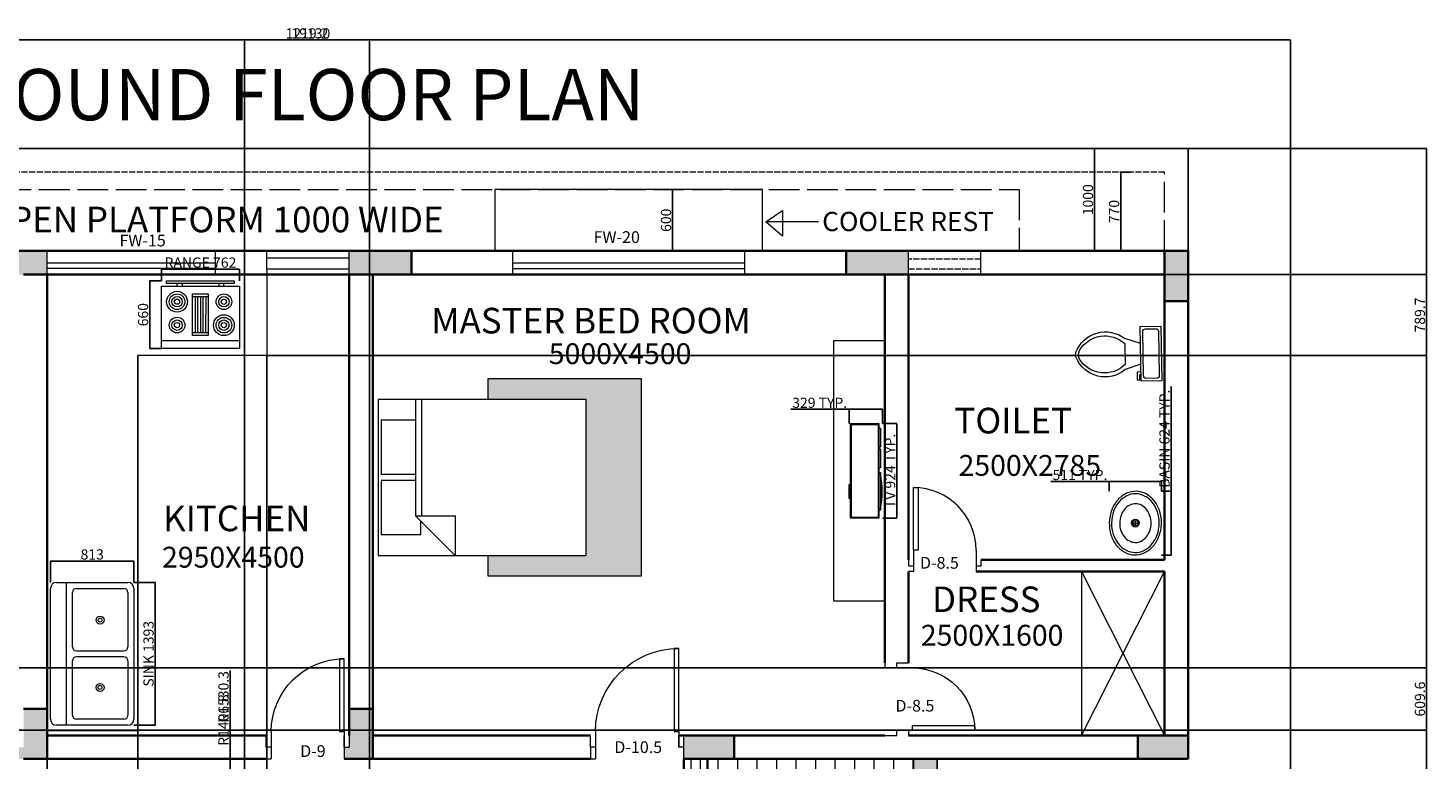
# Model space of a CAD drawing. Units: millimetres. Extents: x -17016 to 4866, y -18325 to 4338.
# Tile 5 of 5: x -8803 to 4866, y -2799 to 4338. Entities that reach past the tile are written whole.
import ezdxf

# ---------------------------------------------------------------- set-up
doc = ezdxf.new("R2010")
doc.units = ezdxf.units.MM
doc.header["$LTSCALE"] = 5
doc.linetypes.add('ACAD_ISO02W100', pattern=[15, 12, -3])
for name, color, linetype, lineweight in [('A-ANNO-DIMS', 2, 'Continuous', 18), ('A-ANNO-IDEN', 3, 'Continuous', 18), ('A-ANNO-SYMB', 7, 'Continuous', 18), ('A-ANNO-TEXT', 7, 'Continuous', 25), ('A-AREA-IDEN', 7, 'Continuous', 25), ('A-COLS', 7, 'Continuous', 35), ('A-COLS-PATT', 252, 'Continuous', 13), ('A-DOOR', 3, 'Continuous', 18), ('A-EQPM', 9, 'Continuous', 18), ('A-FLOR-CASE', 8, 'Continuous', 18), ('A-FLOR-FIXT', 9, 'Continuous', 18), ('A-FLOR-OTLN', 8, 'Continuous', 25), ('A-FLOR-PATT', 252, 'Continuous', 13), ('A-FURN', 8, 'Continuous', 18), ('A-GLAZ', 4, 'Continuous', 18), ('A-GLAZ-HIDN', 4, 'ACAD_ISO02W100', 18), ('A-ROOF', 8, 'Continuous', 18), ('A-ROOF-OVHD', 8, 'ACAD_ISO02W100', 13), ('A-WALL', 7, 'Continuous', 35)]:
    doc.layers.add(name, color=color, linetype=linetype, lineweight=lineweight)
doc.styles.get("Standard").update_dxf_attribs({"font": 'arial.ttf'})
doc.dimstyles.new('Copy of ISO-25', dxfattribs={"dimtxt": 100, "dimasz": 2.5, "dimexe": 1.25, "dimexo": 0.625, "dimtad": 1, "dimdec": 0, "dimtxsty": 'Standard', "dimcen": 2.5, "dimadec": 0, "dimazin": 0, "dimtfac": 1, "dimtdec": 0, "dimtmove": 0, "dimatfit": 3, "dimfxl": 1, "dimarcsym": 0})

# ---------------------------------------------------------------- blocks, each defined once
blk = doc.blocks.new('*U11')
for p, q in [((0, 0), (0, -6)), ((28, 0), (28, -6))]:
    blk.add_line(p, q)
blk.add_lwpolyline([(0, 0), (0, 28), (1.75, 28), (1.75, 0)], close=True)
blk.add_arc((0, 0), 28, 0, 90)
blk = doc.blocks.new('*U2')
for p, q in [((0, 0), (0, -6)), ((32, 0), (32, -6))]:
    blk.add_line(p, q)
blk.add_lwpolyline([(0, 0), (0, 32), (1.75, 32), (1.75, 0)], close=True)
blk.add_arc((0, 0), 32, 0, 90)
blk = doc.blocks.new('*U3')
for p, q in [((0, 0), (0, -6)), ((24, 0), (24, -6))]:
    blk.add_line(p, q)
blk.add_lwpolyline([(0, 0), (0, 24), (1.75, 24), (1.75, 0)], close=True)
blk.add_arc((0, 0), 24, 0, 90)
blk = doc.blocks.new('Bed - Queen')
for p, q in [((0, -80.00003), (0, 0)), ((0, 0), (59.99999, 0)), ((59.99999, 0), (59.99999, -80.00003)), ((7.99999, -1.2), (28.79998, -1.2)), ((7.99999, -14.4), (7.99999, -1.2)), ((28.79998, -1.2), (28.79998, -14.4)), ((31.19999, -1.2), (51.99999, -1.2)), ((31.19999, -14.4), (31.19999, -1.2)), ((51.99999, -1.2), (51.99999, -16.4)), ((0, -14.4), (44.8, -14.4)), ((59.99999, -29.6), (44.8, -14.4)), ((44.8, -14.4), (44.8, -29.6)), ((44.8, -16.8), (0, -16.8)), ((51.99999, -16.4), (46.79936, -16.4)), ((44.8, -29.6), (59.99999, -29.6)), ((59.99999, -80.00003), (0, -80.00003))]:
    blk.add_line(p, q)
blk = doc.blocks.new('Entertainment Center')
for p, q in [((-4, 0), (-5, -1)), ((4, 0), (-4, 0)), ((5, -1), (4, 0)), ((-17, -19), (-17, -1)), ((-17, -1), (43, -1)), ((-16.5, -18.5), (-16.5, -1.5)), ((-16.5, -1.5), (42.5, -1.5)), ((42.5, -1.5), (42.5, -18.5)), ((43, -1), (43, -19)), ((43, -19), (-17, -19)), ((42.5, -18.5), (-16.5, -18.5)), ((-12, -20), (-12, -19)), ((12, -20), (-12, -20)), ((12, -19), (12, -20)), ((15, -20), (15, -19)), ((27, -20), (15, -20)), ((27, -19), (27, -20)), ((28, -20), (28, -19)), ((40, -20), (28, -20)), ((40, -19), (40, -20))]:
    blk.add_line(p, q)
blk.add_arc((0, 40), 61, 259.6111, 280.3889)
blk = doc.blocks.new('*U13')
for p, q in [((9.5, -6), (9.5, -2)), ((-10, -8.5), (-8, -8.5)), ((-10, -9.5), (-10, -8.5)), ((-7, -9.5), (-10, -9.5)), ((-8, -8.5), (-8, -8)), ((-7, -8), (-7, -9.5)), ((-4, -8), (-6, -14)), ((4, -8), (6, -14)), ((4, -14), (-4, -14))]:
    blk.add_line(p, q)
blk.add_lwpolyline([(10.5, -8), (10.5, 0), (-10.5, 0), (-10.5, -8)], close=True)
for points in [[(-9.5, -2), (-9.5, -6)], [(8.5, -1), (-8.5, -1)], [(-8.5, -7), (8.5, -7)]]:
    blk.add_lwpolyline(points)
for centre, radius, start, end in [((-8.62, -1.88), 0.884, 81.8699, 188.1301), ((8.62, -1.88), 0.884, 351.8699, 98.1301), ((-8.62, -6.12), 0.884, 171.8699, 278.1301), ((8.62, -6.12), 0.884, 261.8699, 8.1301), ((3.52, -21.58), 12.17, 141.4691, 247.9714), ((4.2, -21.82), 11.33, 136.3677, 238.9468), ((-3.52, -21.58), 12.17, 292.0284, 38.5307), ((-4.2, -21.82), 11.33, 301.053, 43.6321), ((0, -27.88), 4, 245.7318, 294.2682), ((0, -29), 4, 254.8605, 285.1395)]:
    blk.add_arc(centre, radius, start, end)
blk = doc.blocks.new('Sink - Oval top')
for p, q in [((-1, 0), (1, 0)), ((0, 1), (0, -1))]:
    blk.add_line(p, q)
for points in [[(-12.23, 0.39, 0.117634), (-11.46, -3.36, 0.104469), (-8.88, -6.8, 0.090016), (-5.08, -9.07, 0.08192), (-0.32, -10.02, 0.08192), (4.49, -9.38, 0.090016), (8.42, -7.36, 0.104469), (11.22, -4.09, 0.117634), (12.23, -0.39, 0.117634), (11.46, 3.36, 0.104469), (8.88, 6.8, 0.090016), (5.08, 9.07, 0.08192), (0.32, 10.02, 0.08192), (-4.49, 9.38, 0.090016), (-8.42, 7.36, 0.104469), (-11.22, 4.09, 0.117634)], [(-11.29, 0.16, 0.118622), (-10.52, -3.25, 0.104678), (-8.07, -6.36, 0.089562), (-4.54, -8.37, 0.081185), (-0.13, -9.15, 0.081185), (4.3, -8.49, 0.089562), (7.89, -6.58, 0.104678), (10.42, -3.55, 0.118622), (11.29, -0.16, 0.118622), (10.52, 3.25, 0.104678), (8.07, 6.36, 0.089562), (4.54, 8.37, 0.081185), (0.13, 9.15, 0.081185), (-4.3, 8.49, 0.089562), (-7.89, 6.58, 0.104678), (-10.42, 3.55, 0.118622)], [(-7.42, 0.08, 0.118283), (-6.91, -2.17, 0.104607), (-5.29, -4.21, 0.089718), (-2.97, -5.53, 0.081436), (-0.07, -6.04, 0.081436), (2.84, -5.59, 0.089718), (5.2, -4.33, 0.104607), (6.86, -2.32, 0.118283), (7.42, -0.08, 0.118283), (6.91, 2.17, 0.104607), (5.29, 4.21, 0.089718), (2.97, 5.53, 0.081436), (0.07, 6.04, 0.081436), (-2.84, 5.59, 0.089718), (-5.2, 4.33, 0.104607), (-6.86, 2.32, 0.118283)]]:
    blk.add_lwpolyline(points, format="xyb", close=True)
for radius in [1.5, 1]:
    blk.add_circle((0, 0), radius)
blk = doc.blocks.new('*D17')
at = {"layer": 'A-ANNO-DIMS', "color": 0, "lineweight": -2, "ltscale": 5, "transparency": 16777216}
for p, q in [((1837, 3161), (1610, 3161)), ((1611, 2163), (1611, 3158)), ((1932, 2161), (1610, 2161))]:
    blk.add_line(p, q, dxfattribs=at)
at = {"layer": 'A-ANNO-DIMS', "color": 0, "ltscale": 5, "transparency": 16777216}
for points in [[(1611, 3158), (1611, 3158), (1611, 3161)], [(1611, 2163), (1611, 2163), (1611, 2161)]]:
    blk.add_solid(points, dxfattribs=at)
at = {"layer": 'Defpoints', "color": 0, "ltscale": 5, "transparency": 16777216}
for p in [(1611, 3161), (1838, 3161), (1932, 2161)]:
    blk.add_point(p, dxfattribs=at)
at = {"layer": 'A-ANNO-DIMS', "color": 0, "ltscale": 5, "transparency": 16777216, "insert": (1559, 2661), "char_height": 100, "attachment_point": 5, "rotation": 90}
blk.add_mtext('1000', dxfattribs=at)
blk = doc.blocks.new('*D18')
at = {"layer": 'A-ANNO-DIMS', "color": 0, "lineweight": -2, "ltscale": 5, "transparency": 16777216}
for p, q in [((1960, 2931), (1865, 2931)), ((1866, 2928), (1866, 2163)), ((1960, 2161), (1865, 2161))]:
    blk.add_line(p, q, dxfattribs=at)
at = {"layer": 'A-ANNO-DIMS', "color": 0, "ltscale": 5, "transparency": 16777216}
for points in [[(1866, 2928), (1867, 2928), (1866, 2931)], [(1866, 2163), (1867, 2163), (1866, 2161)]]:
    blk.add_solid(points, dxfattribs=at)
at = {"layer": 'Defpoints', "color": 0, "ltscale": 5, "transparency": 16777216}
for p in [(1961, 2931), (1866, 2161), (1961, 2161)]:
    blk.add_point(p, dxfattribs=at)
at = {"layer": 'A-ANNO-DIMS', "color": 0, "ltscale": 5, "transparency": 16777216, "insert": (1814, 2546), "char_height": 100, "attachment_point": 5, "rotation": 90}
blk.add_mtext('770', dxfattribs=at)
blk = doc.blocks.new('*D19')
at = {"layer": 'A-ANNO-DIMS', "color": 0, "lineweight": -2, "ltscale": 5, "transparency": 16777216}
for p, q in [((-2565, 2761), (-2508, 2761)), ((-2509, 2758), (-2509, 2163)), ((-2565, 2161), (-2508, 2161))]:
    blk.add_line(p, q, dxfattribs=at)
at = {"layer": 'A-ANNO-DIMS', "color": 0, "ltscale": 5, "transparency": 16777216}
for points in [[(-2509, 2758), (-2509, 2758), (-2509, 2761)], [(-2509, 2163), (-2509, 2163), (-2509, 2161)]]:
    blk.add_solid(points, dxfattribs=at)
at = {"layer": 'Defpoints', "color": 0, "ltscale": 5, "transparency": 16777216}
for p in [(-2566, 2761), (-2566, 2161), (-2509, 2161)]:
    blk.add_point(p, dxfattribs=at)
at = {"layer": 'A-ANNO-DIMS', "color": 0, "ltscale": 5, "transparency": 16777216, "insert": (-2561, 2461), "char_height": 100, "attachment_point": 5, "rotation": 90}
blk.add_mtext('600', dxfattribs=at)
blk = doc.blocks.new('Range-Oven - 30 in top')
for p, q in [((0, -3), (30, -3)), ((12, -6), (18, -6)), ((13, -20), (13, -6)), ((14, -6), (14, -20)), ((15, -20), (15, -6)), ((16, -6), (16, -20)), ((17, -20), (17, -6)), ((18, -20), (12, -20)), ((6, -24), (6, -25)), ((8, -25), (8, -24)), ((22, -25), (22, -24)), ((24, -24), (24, -25))]:
    blk.add_line(p, q)
for points in [[(0, -24), (0, 0), (30, 0), (30, -24)], [(12, -21), (12, -5), (18, -5), (18, -21)], [(2, -26), (2, -25), (28, -25), (28, -26)]]:
    blk.add_lwpolyline(points, close=True)
for centre, radius in [((6, -9), 4), ((6, -9), 3), ((6, -9), 2), ((6, -9), 1), ((24, -9), 3), ((24, -9), 2), ((24, -9), 1), ((6, -18), 3), ((6, -18), 2), ((24, -18), 4), ((24, -18), 3), ((24, -18), 2), ((6, -18), 1), ((24, -18), 1)]:
    blk.add_circle(centre, radius)
blk = doc.blocks.new('Sink-double - 36 in top')
for p, q in [((-18, -4), (18, -4)), ((-0.75, -18.5), (-0.75, -6.5)), ((0.75, -6.5), (0.75, -18.5))]:
    blk.add_line(p, q)
for points in [[(-16.5, 0), (16.5, 0)], [(-18, -19.5), (-18, -1.5)], [(18, -1.5), (18, -19.5)], [(-16.5, -18.5), (-16.5, -6.5)], [(-15.5, -5.5), (-1.75, -5.5)], [(1.75, -5.5), (15.5, -5.5)], [(16.5, -6.5), (16.5, -18.5)], [(16.5, -21), (-16.5, -21)], [(-1.75, -19.5), (-15.5, -19.5)], [(15.5, -19.5), (1.75, -19.5)]]:
    blk.add_lwpolyline(points)
for centre, radius in [((-8.5, -12.5), 1), ((-8.5, -12.5), 0.5), ((8.5, -12.5), 1), ((8.5, -12.5), 0.5)]:
    blk.add_circle(centre, radius)
for centre, radius, start, end in [((-16.5, -1.5), 1.5, 90, 180), ((16.5, -1.5), 1.5, 0, 90), ((-15.5, -6.5), 1, 90, 180), ((-1.75, -6.5), 1, 0, 90), ((1.75, -6.5), 1, 90, 180), ((15.5, -6.5), 1, 0, 90), ((-16.5, -19.5), 1.5, 180, 270), ((-15.5, -18.5), 1, 180, 270), ((-1.75, -18.5), 1, 270, 0), ((1.75, -18.5), 1, 180, 270), ((15.5, -18.5), 1, 270, 0), ((16.5, -19.5), 1.5, 270, 0)]:
    blk.add_arc(centre, radius, start, end)
blk = doc.blocks.new('WIN-FW20')
for p, q in [((0, 0), (0, 230)), ((2263, 0), (2263, 230)), ((0, 115), (2263, 115)), ((0, 60), (2263, 60))]:
    blk.add_line(p, q)
blk = doc.blocks.new('*D26')
at = {"layer": 'A-ANNO-DIMS', "color": 0, "lineweight": -2, "ltscale": 5, "transparency": 16777216}
for p, q in [((-458, 476), (-319, 476)), ((-320, -446), (-320, 473)), ((-458, -448), (-319, -448))]:
    blk.add_line(p, q, dxfattribs=at)
at = {"layer": 'A-ANNO-DIMS', "color": 0, "ltscale": 5, "transparency": 16777216}
for points in [[(-320, 473), (-320, 473), (-320, 476)], [(-320, -446), (-320, -446), (-320, -448)]]:
    blk.add_solid(points, dxfattribs=at)
at = {"layer": 'Defpoints', "color": 0, "ltscale": 5, "transparency": 16777216}
for p in [(-459, 476), (-320, 476), (-459, -448)]:
    blk.add_point(p, dxfattribs=at)
at = {"layer": 'A-ANNO-DIMS', "color": 0, "ltscale": 5, "transparency": 16777216, "insert": (-372, 14), "char_height": 100, "attachment_point": 5, "rotation": 90}
blk.add_mtext('TV 924 TYP.', dxfattribs=at)
blk = doc.blocks.new('*D27')
at = {"layer": 'A-ANNO-DIMS', "color": 0, "lineweight": -2, "ltscale": 5, "transparency": 16777216}
for p, q in [((-787, 615), (-1355, 615)), ((-787, 477), (-787, 616)), ((-461, 615), (-785, 615)), ((-459, 477), (-459, 616))]:
    blk.add_line(p, q, dxfattribs=at)
at = {"layer": 'A-ANNO-DIMS', "color": 0, "ltscale": 5, "transparency": 16777216}
for points in [[(-785, 615), (-785, 614), (-787, 615)], [(-461, 615), (-461, 614), (-459, 615)]]:
    blk.add_solid(points, dxfattribs=at)
at = {"layer": 'Defpoints', "color": 0, "ltscale": 5, "transparency": 16777216}
for p in [(-787, 615), (-787, 476), (-459, 476)]:
    blk.add_point(p, dxfattribs=at)
at = {"layer": 'A-ANNO-DIMS', "color": 0, "ltscale": 5, "transparency": 16777216, "insert": (-1073, 666), "char_height": 100, "attachment_point": 5}
blk.add_mtext('329 TYP.', dxfattribs=at)
blk = doc.blocks.new('*D28')
at = {"layer": 'A-ANNO-DIMS', "color": 0, "lineweight": -2, "ltscale": 5, "transparency": 16777216}
for p, q in [((2358, -184), (2358, 838)), ((2265, -184), (2360, -184)), ((2358, -805), (2358, -187)), ((2265, -808), (2360, -808))]:
    blk.add_line(p, q, dxfattribs=at)
at = {"layer": 'A-ANNO-DIMS', "color": 0, "ltscale": 5, "transparency": 16777216}
for points in [[(2358, -187), (2359, -187), (2358, -184)], [(2358, -805), (2359, -805), (2358, -808)]]:
    blk.add_solid(points, dxfattribs=at)
at = {"layer": 'Defpoints', "color": 0, "ltscale": 5, "transparency": 16777216}
for p in [(2265, -184), (2358, -184), (2265, -808)]:
    blk.add_point(p, dxfattribs=at)
at = {"layer": 'A-ANNO-DIMS', "color": 0, "ltscale": 5, "transparency": 16777216, "insert": (2306, 328), "char_height": 100, "attachment_point": 5, "rotation": 90}
blk.add_mtext('BASIN 624 TYP.', dxfattribs=at)
blk = doc.blocks.new('*D29')
at = {"layer": 'A-ANNO-DIMS', "color": 0, "lineweight": -2, "ltscale": 5, "transparency": 16777216}
for p, q in [((1753, -91), (1185, -91)), ((1753, -184), (1753, -89)), ((2262, -91), (1756, -91)), ((2265, -184), (2265, -89))]:
    blk.add_line(p, q, dxfattribs=at)
at = {"layer": 'A-ANNO-DIMS', "color": 0, "ltscale": 5, "transparency": 16777216}
for points in [[(1756, -90), (1756, -91), (1753, -91)], [(2262, -90), (2262, -91), (2265, -91)]]:
    blk.add_solid(points, dxfattribs=at)
at = {"layer": 'Defpoints', "color": 0, "ltscale": 5, "transparency": 16777216}
for p in [(1753, -91), (1753, -184), (2265, -184)]:
    blk.add_point(p, dxfattribs=at)
at = {"layer": 'A-ANNO-DIMS', "color": 0, "ltscale": 5, "transparency": 16777216, "insert": (1468, -39), "char_height": 100, "attachment_point": 5}
blk.add_mtext('511 TYP.', dxfattribs=at)
blk = doc.blocks.new('*D42')
at = {"layer": 'A-ANNO-DIMS', "color": 0, "lineweight": -2, "ltscale": 5, "transparency": 16777216}
for p, q in [((-7500, 1869), (-7500, 1984)), ((-6740, 1983), (-7497, 1983)), ((-6738, 1869), (-6738, 1984))]:
    blk.add_line(p, q, dxfattribs=at)
at = {"layer": 'A-ANNO-DIMS', "color": 0, "ltscale": 5, "transparency": 16777216}
for points in [[(-7497, 1983), (-7497, 1983), (-7500, 1983)], [(-6740, 1983), (-6740, 1982), (-6738, 1983)]]:
    blk.add_solid(points, dxfattribs=at)
at = {"layer": 'Defpoints', "color": 0, "ltscale": 5, "transparency": 16777216}
for p in [(-7500, 1983), (-7500, 1869), (-6738, 1868)]:
    blk.add_point(p, dxfattribs=at)
at = {"layer": 'A-ANNO-DIMS', "color": 0, "ltscale": 5, "transparency": 16777216, "insert": (-7119, 2035), "char_height": 100, "attachment_point": 5, "rotation": 359.9761}
blk.add_mtext('RANGE 762', dxfattribs=at)
blk = doc.blocks.new('*D43')
at = {"layer": 'A-ANNO-DIMS', "color": 0, "lineweight": -2, "ltscale": 5, "transparency": 16777216}
for p, q in [((-7500, 1869), (-7615, 1869)), ((-7614, 1866), (-7614, 1211)), ((-7501, 1208), (-7616, 1208))]:
    blk.add_line(p, q, dxfattribs=at)
at = {"layer": 'A-ANNO-DIMS', "color": 0, "ltscale": 5, "transparency": 16777216}
for points in [[(-7615, 1866), (-7614, 1866), (-7614, 1869)], [(-7615, 1211), (-7614, 1211), (-7614, 1208)]]:
    blk.add_solid(points, dxfattribs=at)
at = {"layer": 'Defpoints', "color": 0, "ltscale": 5, "transparency": 16777216}
for p in [(-7500, 1869), (-7614, 1208), (-7500, 1208)]:
    blk.add_point(p, dxfattribs=at)
at = {"layer": 'A-ANNO-DIMS', "color": 0, "ltscale": 5, "transparency": 16777216, "insert": (-7666, 1539), "char_height": 100, "attachment_point": 5, "rotation": 89.9761}
blk.add_mtext('660', dxfattribs=at)
blk = doc.blocks.new('*D44')
at = {"layer": 'A-ANNO-DIMS', "color": 0, "lineweight": -2, "ltscale": 5, "transparency": 16777216}
for p, q in [((-7769, -1076), (-7559, -1076)), ((-7561, -2466), (-7561, -1078)), ((-7769, -2469), (-7559, -2469))]:
    blk.add_line(p, q, dxfattribs=at)
at = {"layer": 'A-ANNO-DIMS', "color": 0, "ltscale": 5, "transparency": 16777216}
for points in [[(-7561, -1078), (-7560, -1078), (-7561, -1076)], [(-7561, -2466), (-7560, -2466), (-7561, -2469)]]:
    blk.add_solid(points, dxfattribs=at)
at = {"layer": 'Defpoints', "color": 0, "ltscale": 5, "transparency": 16777216}
for p in [(-7770, -1076), (-7561, -1076), (-7770, -2469)]:
    blk.add_point(p, dxfattribs=at)
at = {"layer": 'A-ANNO-DIMS', "color": 0, "ltscale": 5, "transparency": 16777216, "insert": (-7613, -1772), "char_height": 100, "attachment_point": 5, "rotation": 90}
blk.add_mtext('SINK 1393', dxfattribs=at)
blk = doc.blocks.new('*D45')
at = {"layer": 'A-ANNO-DIMS', "color": 0, "lineweight": -2, "ltscale": 5, "transparency": 16777216}
for p, q in [((-8582, -1075), (-8582, -865)), ((-7772, -867), (-8580, -867)), ((-7770, -1075), (-7770, -865))]:
    blk.add_line(p, q, dxfattribs=at)
at = {"layer": 'A-ANNO-DIMS', "color": 0, "ltscale": 5, "transparency": 16777216}
for points in [[(-8580, -866), (-8580, -867), (-8582, -867)], [(-7772, -866), (-7772, -867), (-7770, -867)]]:
    blk.add_solid(points, dxfattribs=at)
at = {"layer": 'Defpoints', "color": 0, "ltscale": 5, "transparency": 16777216}
for p in [(-8582, -867), (-8582, -1076), (-7770, -1076)]:
    blk.add_point(p, dxfattribs=at)
at = {"layer": 'A-ANNO-DIMS', "color": 0, "ltscale": 5, "transparency": 16777216, "insert": (-8176, -815), "char_height": 100, "attachment_point": 5}
blk.add_mtext('813', dxfattribs=at)
blk = doc.blocks.new('*D46')
at = {"layer": 'A-ANNO-DIMS', "color": 0, "lineweight": -2, "ltscale": 5, "transparency": 16777216}
for p, q in [((-15606, 3162), (-15606, 4222)), ((-15604, 4221), (3521, 4221)), ((3524, 3162), (3524, 4222))]:
    blk.add_line(p, q, dxfattribs=at)
at = {"layer": 'A-ANNO-DIMS', "color": 0, "ltscale": 5, "transparency": 16777216}
for points in [[(-15604, 4221), (-15604, 4220), (-15606, 4221)], [(3521, 4221), (3521, 4220), (3524, 4221)]]:
    blk.add_solid(points, dxfattribs=at)
at = {"layer": 'Defpoints', "color": 0, "ltscale": 5, "transparency": 16777216}
for p in [(3524, 4221), (-15606, 3161), (3524, 3161)]:
    blk.add_point(p, dxfattribs=at)
at = {"layer": 'A-ANNO-DIMS', "color": 0, "ltscale": 5, "transparency": 16777216, "insert": (-6041, 4272), "char_height": 100, "attachment_point": 5}
blk.add_mtext('19130', dxfattribs=at)
blk = doc.blocks.new('*D47')
at = {"layer": 'A-ANNO-DIMS', "color": 0, "lineweight": -2, "ltscale": 5, "transparency": 16777216}
for p, q in [((3524, 3161), (4853, 3161)), ((4852, 3158), (4852, -17248)), ((-3160, -17251), (4853, -17251))]:
    blk.add_line(p, q, dxfattribs=at)
at = {"layer": 'A-ANNO-DIMS', "color": 0, "ltscale": 5, "transparency": 16777216}
for points in [[(4851, 3158), (4852, 3158), (4852, 3161)], [(4851, -17248), (4852, -17248), (4852, -17251)]]:
    blk.add_solid(points, dxfattribs=at)
at = {"layer": 'Defpoints', "color": 0, "ltscale": 5, "transparency": 16777216}
for p in [(3524, 3161), (-3160, -17251), (4852, -17251)]:
    blk.add_point(p, dxfattribs=at)
at = {"layer": 'A-ANNO-DIMS', "color": 0, "ltscale": 5, "transparency": 16777216, "insert": (4800, -7045), "char_height": 100, "attachment_point": 5, "rotation": 90}
blk.add_mtext('20412', dxfattribs=at)
blk = doc.blocks.new('*D52')
at = {"layer": 'A-ANNO-DIMS', "color": 0, "lineweight": -2, "ltscale": 5, "transparency": 16777216}
for p, q in [((-12346, -1910), (4853, -1910)), ((4852, -2517), (4852, -1912)), ((-12346, -2519), (4853, -2519))]:
    blk.add_line(p, q, dxfattribs=at)
at = {"layer": 'A-ANNO-DIMS', "color": 0, "ltscale": 5, "transparency": 16777216}
for points in [[(4851, -1912), (4852, -1912), (4852, -1910)], [(4851, -2517), (4852, -2517), (4852, -2519)]]:
    blk.add_solid(points, dxfattribs=at)
at = {"layer": 'Defpoints', "color": 0, "ltscale": 5, "transparency": 16777216}
for p in [(-12346, -1910), (4852, -1910), (-12346, -2519)]:
    blk.add_point(p, dxfattribs=at)
at = {"layer": 'A-ANNO-DIMS', "color": 0, "ltscale": 5, "transparency": 16777216, "insert": (4800, -2214), "char_height": 100, "attachment_point": 5, "rotation": 90}
blk.add_mtext('609.6', dxfattribs=at)
blk = doc.blocks.new('*D53')
at = {"layer": 'A-ANNO-DIMS', "color": 0, "lineweight": -2, "ltscale": 5, "transparency": 16777216}
for p, q in [((-6689, -11408), (-6689, 4222)), ((-6686, 4221), (-5472, 4221)), ((-5470, -11408), (-5470, 4222))]:
    blk.add_line(p, q, dxfattribs=at)
at = {"layer": 'A-ANNO-DIMS', "color": 0, "ltscale": 5, "transparency": 16777216}
for points in [[(-6686, 4221), (-6686, 4220), (-6689, 4221)], [(-5472, 4221), (-5472, 4220), (-5470, 4221)]]:
    blk.add_solid(points, dxfattribs=at)
at = {"layer": 'Defpoints', "color": 0, "ltscale": 5, "transparency": 16777216}
for p in [(-5470, 4221), (-6689, -11409), (-5470, -11409)]:
    blk.add_point(p, dxfattribs=at)
at = {"layer": 'A-ANNO-DIMS', "color": 0, "ltscale": 5, "transparency": 16777216, "insert": (-6079, 4272), "char_height": 100, "attachment_point": 5}
blk.add_mtext('1219.2', dxfattribs=at)
blk = doc.blocks.new('*D54')
at = {"layer": 'A-ANNO-DIMS', "color": 0, "lineweight": -2, "ltscale": 5, "transparency": 16777216}
for p, q in [((-7730, 1141), (-7730, -18312)), ((-6472, 1141), (-6472, -18312)), ((-7727, -18311), (-6475, -18311))]:
    blk.add_line(p, q, dxfattribs=at)
at = {"layer": 'A-ANNO-DIMS', "color": 0, "ltscale": 5, "transparency": 16777216}
for points in [[(-7727, -18310), (-7727, -18311), (-7730, -18311)], [(-6475, -18310), (-6475, -18311), (-6472, -18311)]]:
    blk.add_solid(points, dxfattribs=at)
at = {"layer": 'Defpoints', "color": 0, "ltscale": 5, "transparency": 16777216}
for p in [(-7730, 1141), (-6472, 1141), (-6472, -18311)]:
    blk.add_point(p, dxfattribs=at)
at = {"layer": 'A-ANNO-DIMS', "color": 0, "ltscale": 5, "transparency": 16777216, "insert": (-7101, -18259), "char_height": 100, "attachment_point": 5}
blk.add_mtext('1257.7', dxfattribs=at)
blk = doc.blocks.new('*D55')
at = {"layer": 'A-ANNO-DIMS', "color": 0, "lineweight": -2, "ltscale": 5, "transparency": 16777216}
for p, q in [((-6472, 1931), (4853, 1931)), ((4852, 1928), (4852, 1144)), ((-6472, 1141), (4853, 1141))]:
    blk.add_line(p, q, dxfattribs=at)
at = {"layer": 'A-ANNO-DIMS', "color": 0, "ltscale": 5, "transparency": 16777216}
for points in [[(4851, 1928), (4852, 1928), (4852, 1931)], [(4851, 1144), (4852, 1144), (4852, 1141)]]:
    blk.add_solid(points, dxfattribs=at)
at = {"layer": 'Defpoints', "color": 0, "ltscale": 5, "transparency": 16777216}
for p in [(-6472, 1931), (-6472, 1141), (4852, 1141)]:
    blk.add_point(p, dxfattribs=at)
at = {"layer": 'A-ANNO-DIMS', "color": 0, "ltscale": 5, "transparency": 16777216, "insert": (4800, 1536), "char_height": 100, "attachment_point": 5, "rotation": 90}
blk.add_mtext('789.7', dxfattribs=at)
blk = doc.blocks.new('*D56')
at = {"layer": 'A-ANNO-DIMS', "color": 0, "lineweight": -2, "ltscale": 5, "transparency": 16777216}
for p, q in [((-8616, -2525), (-8616, -18312)), ((-7730, -2525), (-7730, -18312)), ((-8614, -18311), (-7732, -18311))]:
    blk.add_line(p, q, dxfattribs=at)
at = {"layer": 'A-ANNO-DIMS', "color": 0, "ltscale": 5, "transparency": 16777216}
for points in [[(-8614, -18310), (-8614, -18311), (-8616, -18311)], [(-7732, -18310), (-7732, -18311), (-7730, -18311)]]:
    blk.add_solid(points, dxfattribs=at)
at = {"layer": 'Defpoints', "color": 0, "ltscale": 5, "transparency": 16777216}
for p in [(-8616, -2525), (-7730, -2525), (-7730, -18311)]:
    blk.add_point(p, dxfattribs=at)
at = {"layer": 'A-ANNO-DIMS', "color": 0, "ltscale": 5, "transparency": 16777216, "insert": (-8173, -18259), "char_height": 100, "attachment_point": 5}
blk.add_mtext('886.5', dxfattribs=at)
blk = doc.blocks.new('*D59')
at = {"layer": 'A-ANNO-DIMS', "color": 0, "lineweight": -2, "ltscale": 5, "transparency": 16777216}
for p, q in [((-6829, -1936), (-6829, -3108)), ((-6829, -4641), (-6829, -3111))]:
    blk.add_line(p, q, dxfattribs=at)
at = {"layer": 'A-ANNO-DIMS', "color": 0, "ltscale": 5, "transparency": 16777216}
blk.add_solid([(-6829, -3108), (-6829, -3108), (-6829, -3111)], dxfattribs=at)
at = {"layer": 'Defpoints', "color": 0, "ltscale": 5, "transparency": 16777216}
for p in [(-6829, -3111), (-6829, -4641)]:
    blk.add_point(p, dxfattribs=at)
at = {"layer": 'A-ANNO-DIMS', "color": 0, "ltscale": 5, "transparency": 16777216, "insert": (-6881, -2192), "char_height": 100, "attachment_point": 5, "rotation": 90}
blk.add_mtext('R1530.3', dxfattribs=at)
blk = doc.blocks.new('*D60')
at = {"layer": 'A-ANNO-DIMS', "color": 0, "lineweight": -2, "ltscale": 5, "transparency": 16777216}
for p, q in [((-6829, -2163), (-6829, -3261)), ((-6829, -4670), (-6829, -3263))]:
    blk.add_line(p, q, dxfattribs=at)
at = {"layer": 'A-ANNO-DIMS', "color": 0, "ltscale": 5, "transparency": 16777216}
blk.add_solid([(-6829, -3261), (-6829, -3261), (-6829, -3263)], dxfattribs=at)
at = {"layer": 'Defpoints', "color": 0, "ltscale": 5, "transparency": 16777216}
for p in [(-6829, -3263), (-6829, -4670)]:
    blk.add_point(p, dxfattribs=at)
at = {"layer": 'A-ANNO-DIMS', "color": 0, "ltscale": 5, "transparency": 16777216, "insert": (-6881, -2419), "char_height": 100, "attachment_point": 5, "rotation": 90}
blk.add_mtext('R1406.8', dxfattribs=at)

msp = doc.modelspace()

# ---------------------------------------------------------------- hatches: boundary and pattern name
at = {"layer": 'A-COLS-PATT', "ltscale": 5}
h = msp.add_hatch(color=256, dxfattribs=at)
h.dxf.hatch_style = 1
h.paths.add_polyline_path([(2523.62, 2160.89), (2293.62, 2160.89), (2293.62, 1930.89), (2293.62, 1670.89), (2523.62, 1670.89)])
h.paths.add_polyline_path([(-14116.35, 2160.89), (-14606.38, 2160.89), (-14606.38, 1930.89), (-14116.35, 1930.89)])
h = msp.add_hatch(color=256, dxfattribs=at)
h.dxf.hatch_style = 1
h.paths.add_polyline_path([(-8616.38, 2160.89), (-9107.57, 2160.89), (-9107.57, 1930.89), (-8846.38, 1930.89), (-8616.38, 1930.89)])
at = {"layer": 'A-COLS-PATT'}
h = msp.add_hatch(color=256, dxfattribs=at)
h.dxf.hatch_style = 1
h.paths.add_polyline_path([(-5059.38, 2160.89), (-5666.38, 2160.89), (-5666.38, 1930.89), (-5436.38, 1930.89), (-5059.38, 1930.89)])
h.paths.add_polyline_path([(-206.38, 2160.89), (-813.57, 2160.89), (-813.57, 1930.89), (-436.38, 1930.89), (-206.38, 1930.89)])
at = {"layer": 'A-COLS-PATT', "ltscale": 5}
h = msp.add_hatch(color=256, dxfattribs=at)
h.dxf.hatch_style = 1
h.paths.add_polyline_path([(2523.62, -2569.11), (2033.62, -2569.11), (2033.62, -2799.11), (2523.62, -2799.11)])
h.paths.add_polyline_path([(-1909.18, -2569.11), (-2399.18, -2569.11), (-2399.18, -2799.11), (-1909.18, -2799.11)])
h.paths.add_polyline_path([(-5436.38, -2309.11), (-5666.38, -2309.11), (-5666.38, -2569.11), (-5666.38, -2684.11), (-5716.38, -2684.11), (-5716.38, -2799.11), (-5436.38, -2799.11)])
h.paths.add_polyline_path([(-8616.38, -2309.11), (-8846.38, -2309.11), (-8846.38, -2569.11), (-8846.38, -2684.11), (-8896.38, -2684.11), (-8896.38, -2799.11), (-8846.38, -2799.11), (-8616.38, -2799.11)])
at = {"layer": 'A-FLOR-PATT'}
h = msp.add_hatch(dxfattribs=at)
h.set_pattern_fill('ANSI38', color=256, scale=25)
h.set_pattern_definition([(45, (-20162.07, -7174.37), (-56.1266, 56.1266), []), (135, (-20162.07, -7174.37), (-168.3798, 56.1266), [198.4375, -119.0625])])
h.paths.add_polyline_path([(-1358.58, -10190.51), (-396.23, -10190.51), (-396.23, -9990.51), (-1896.23, -9990.51), (-1896.23, -11914.51), (-396.23, -11914.51), (-396.23, -11714.51), (-1358.58, -11714.51)])
h.paths.add_polyline_path([(-10262.12, -9990.51), (-11762.12, -9990.51), (-11762.12, -10190.51), (-10799.77, -10190.51), (-10799.77, -11714.51), (-11762.12, -11714.51), (-11762.12, -11914.51), (-10262.12, -11914.51)])
h.paths.add_polyline_path([(-9722.08, 912.47), (-11222.08, 912.47), (-11222.08, 712.47), (-10260.08, 712.47), (-10260.08, -811.53), (-11222.08, -811.53), (-11222.08, -1011.53), (-9722.08, -1011.53)])
h.paths.add_polyline_path([(-2814.18, 912.47), (-4314.18, 912.47), (-4314.18, 712.47), (-3352.18, 712.47), (-3352.18, -811.53), (-4314.18, -811.53), (-4314.18, -1011.53), (-2814.18, -1011.53)])
h = msp.add_hatch(dxfattribs=at)
h.set_pattern_fill('ANGLE', color=256, scale=25)
h.set_pattern_definition([(0, (-20162.07, -7174.37), (0, 174.625), [127, -47.625]), (90, (-20162.07, -7174.37), (-174.625, 1e-14), [127, -47.625])])
h.paths.add_polyline_path([(72.82, -2799.11), (-157.18, -2799.11), (-157.18, -7299.11), (72.82, -7299.11)])
h.paths.add_polyline_path([(-12231.38, -2799.11), (-12461.38, -2799.11), (-12461.38, -7299.11), (-12231.38, -7299.11)])
h = msp.add_hatch(dxfattribs=at)
h.set_pattern_fill('SQUARE', color=256, scale=60)
h.set_pattern_definition([(0, (-20162.07, -7174.37), (0, 190.5), [190.5, -190.5]), (90, (-20162.07, -7174.37), (-190.5, 1e-14), [190.5, -190.5])])
h.paths.add_polyline_path([(-157.18, -2799.11), (-436.38, -2799.11), (-2169.18, -2799.11), (-2169.18, -4439.51), (-2169.18, -5658.71), (-2169.18, -7299.11), (-157.18, -7299.11)])
h.paths.add_polyline_path([(-9989.18, -4439.51), (-9989.18, -2799.11), (-12231.38, -2799.11), (-12231.38, -7299.11), (-9989.18, -7299.11), (-9989.18, -5658.71)])

# ---------------------------------------------------------------- linework, layer by layer
at = {"layer": 'A-ANNO-SYMB', "ltscale": 5}
msp.add_lwpolyline([(-1084.49, 2445.58), (-1599.82, 2443.94), (-1437.14, 2555.4), (-1437.14, 2304.62), (-1599.82, 2443.94)], dxfattribs=at)
at = {"layer": 'A-COLS'}
for p, q in [((-5059.38, 1930.89), (-5059.38, 2160.89)), ((-813.57, 1930.89), (-813.57, 2160.89)), ((-5436.38, 1930.89), (-5666.38, 1930.89)), ((-436.38, 1930.89), (-166.11, 1930.89))]:
    msp.add_line(p, q, dxfattribs=at)
at = {"layer": 'A-COLS', "ltscale": 5}
for p, q in [((2293.62, 1930.89), (2293.62, 2160.89)), ((-8846.38, 1930.89), (-8616.38, 1930.89)), ((2293.62, 1670.89), (2523.62, 1670.89)), ((-8616.38, -2309.11), (-8846.38, -2309.11)), ((-5436.38, -2309.11), (-5666.38, -2309.11)), ((-1909.18, -2799.11), (-1909.18, -2569.11)), ((2033.62, -2569.11), (2033.62, -2799.11))]:
    msp.add_line(p, q, dxfattribs=at)
at = {"layer": 'A-DOOR'}
for p, q in [((-206.38, -854.11), (-206.38, -911.61)), ((-206.38, -911.61), (-156.38, -911.61)), ((-156.38, -911.61), (-156.38, -969.11)), ((453.22, -911.61), (503.22, -911.61)), ((453.22, -911.61), (453.22, -969.11)), ((503.22, -911.61), (503.22, -854.11)), ((-156.38, -969.11), (-206.38, -969.11)), ((-436.38, -1859.51), (-436.38, -1909.51)), ((-321.38, -1909.51), (-436.38, -1909.51)), ((-321.38, -1909.51), (-321.38, -1859.51)), ((-321.38, -1859.51), (-206.38, -1859.51)), ((-6477.58, -2684.11), (-6477.58, -2569.11)), ((-5716.38, -2684.11), (-5716.38, -2569.11)), ((-5666.38, -2569.11), (-5666.38, -2684.11)), ((-3311.98, -2684.11), (-3311.98, -2569.11)), ((-2449.18, -2684.11), (-2449.18, -2569.11)), ((-2399.18, -2799.11), (-2399.18, -2569.11)), ((-436.38, -2569.11), (-321.38, -2569.11)), ((-321.38, -2569.11), (-321.38, -2519.11)), ((-206.38, -2519.11), (-206.38, -2569.11)), ((-6427.58, -2684.11), (-6477.58, -2684.11)), ((-6427.58, -2684.11), (-6427.58, -2799.11)), ((-5716.38, -2684.11), (-5716.38, -2799.11)), ((-5716.38, -2684.11), (-5666.38, -2684.11)), ((-3261.98, -2684.11), (-3311.98, -2684.11)), ((-3311.98, -2684.11), (-3311.98, -2799.11)), ((-3261.98, -2684.11), (-3261.98, -2799.11)), ((-2399.18, -2684.11), (-2449.18, -2684.11)), ((-6477.58, -2799.11), (-6427.58, -2799.11)), ((-3311.98, -2799.11), (-3261.98, -2799.11))]:
    msp.add_line(p, q, dxfattribs=at)
at = {"layer": 'A-FLOR-CASE'}
for p, q in [((-6472.15, 1930.89), (-6472.15, 1141.22)), ((-6472.15, 1141.22), (-7729.85, 1141.22)), ((-7729.85, 1141.22), (-7729.85, -2524.75)), ((1483.4, -969.11), (1483.4, -2569.11)), ((1483.4, -2569.11), (2293.62, -969.11)), ((1483.4, -969.11), (2293.62, -2569.11)), ((-7729.85, -2524.75), (-8616.38, -2524.75))]:
    msp.add_line(p, q, dxfattribs=at)
at = {"layer": 'A-FLOR-OTLN'}
for p, q in [((2523.62, 3160.89), (-14606.38, 3160.89)), ((-157.18, -2799.11), (-157.18, -7299.11)), ((72.82, -2799.11), (72.82, -7299.11))]:
    msp.add_line(p, q, dxfattribs=at)
at = {"layer": 'A-FLOR-OTLN', "ltscale": 5}
for p, q in [((2523.62, 3160.89), (3523.62, 3160.89)), ((2523.62, 2160.89), (2523.62, 3160.89)), ((3523.62, 3160.89), (3523.62, -2799.11)), ((3523.62, -2799.11), (3523.62, -3799.11))]:
    msp.add_line(p, q, dxfattribs=at)
at = {"layer": 'A-FLOR-PATT'}
msp.add_lwpolyline([(-4314.18, -811.53), (-4314.18, -1011.53), (-2814.18, -1011.53), (-2814.18, 912.47), (-4314.18, 912.47), (-4314.18, 712.47)], dxfattribs=at)
at = {"layer": 'A-FURN'}
msp.add_lwpolyline([(-436.38, -1258.32), (-936.38, -1258.32), (-936.38, 1287.26), (-436.38, 1287.26)], dxfattribs=at)
at = {"layer": 'A-GLAZ'}
for p, q in [((-8616.38, 1930.89), (-8616.38, 2160.89)), ((-6976.5, 2160.89), (-6976.5, 1930.89)), ((-6472.15, 1970.15), (-6472.15, 2160.89)), ((-6472.15, 2094.09), (-5666.38, 2094.09)), ((-5666.38, 1930.89), (-5666.38, 2160.89)), ((-206.38, 1930.89), (-206.38, 2160.89)), ((500.22, 1930.89), (500.22, 2160.89)), ((-8616.38, 2045.89), (-6976.5, 2045.89)), ((-8616.38, 1991.52), (-6976.5, 1991.52)), ((-6472.15, 1985.82), (-5666.38, 1985.82)), ((-6472.15, 1970.15), (-6472.15, 1930.89)), ((-2331.16, -2799.11), (-2331.16, -3889.51)), ((-2239.42, -2799.11), (-2239.42, -3889.51))]:
    msp.add_line(p, q, dxfattribs=at)
at = {"layer": 'A-GLAZ-HIDN'}
for p, q in [((500.22, 2081.77), (-206.38, 2081.77)), ((-206.38, 1985.53), (500.22, 1985.53))]:
    msp.add_line(p, q, dxfattribs=at)
at = {"layer": 'A-ROOF', "ltscale": 5}
for p, q in [((-4242.38, 2160.89), (-4242.38, 2760.89)), ((-1631.15, 2760.89), (-4242.38, 2760.89)), ((-1631.15, 2160.89), (-1631.15, 2760.89))]:
    msp.add_line(p, q, dxfattribs=at)
at = {"layer": 'A-ROOF-OVHD'}
msp.add_line((2293.62, 2930.89), (-13106.38, 2930.89), dxfattribs=at)
at = {"layer": 'A-ROOF-OVHD', "ltscale": 5}
for p, q in [((2293.62, 2160.89), (2293.62, 2930.89)), ((-13570.85, 2760.89), (874.92, 2760.89)), ((874.92, 2760.89), (874.92, 2160.89))]:
    msp.add_line(p, q, dxfattribs=at)
at = {"layer": 'A-WALL'}
for p, q in [((2523.62, 2160.89), (-14606.38, 2160.89)), ((2523.62, 2160.89), (2523.62, -2799.11)), ((-8616.38, 1930.89), (-8616.38, -2799.11)), ((-5666.38, 1930.89), (-8616.38, 1930.89)), ((-5666.38, 1930.89), (-5666.38, -2569.11)), ((-5436.38, 1930.89), (-5436.38, -2799.11)), ((-436.38, 1930.89), (-5436.38, 1930.89)), ((-436.38, 1930.89), (-436.38, -1859.51)), ((2293.62, 1930.89), (-206.38, 1930.89)), ((-206.38, 1930.89), (-206.38, -854.11)), ((2293.62, 1930.89), (2293.62, -854.11)), ((2293.62, -854.11), (503.22, -854.11)), ((-206.38, -969.11), (-206.38, -1859.51)), ((2293.62, -969.11), (453.22, -969.11)), ((2293.62, -969.11), (2293.62, -2569.11)), ((-6477.58, -2569.11), (-8616.38, -2569.11)), ((-3311.98, -2569.11), (-5436.38, -2569.11)), ((-436.38, -2569.11), (-2449.18, -2569.11)), ((2523.62, -2569.11), (-206.38, -2569.11)), ((-6477.58, -2799.11), (-8846.38, -2799.11)), ((-3311.98, -2799.11), (-5716.38, -2799.11)), ((-436.38, -2799.11), (-2399.18, -2799.11)), ((-2399.18, -2799.11), (-2399.18, -4389.51)), ((-2169.18, -2799.11), (-2169.18, -4439.51)), ((2523.62, -2799.11), (-436.38, -2799.11))]:
    msp.add_line(p, q, dxfattribs=at)

# ---------------------------------------------------------------- block references
at = {"layer": 'A-DOOR', "yscale": 25.4, "zscale": 25.4}
for name, p, xscale in [('*U3', (-156.38, -759.21), 25.4), ('*U2', (-2449.18, -2531.71), -25.4), ('*U11', (-5716.38, -2531.71), -25.4)]:
    msp.add_blockref(name, p, dxfattribs=dict(at, xscale=xscale))
at = {"layer": 'A-DOOR', "xscale": -25.4, "yscale": 25.4, "zscale": 25.4, "rotation": 270}
msp.add_blockref('*U3', (-168.98, -2519.11), dxfattribs=at)
at = {"layer": 'A-EQPM', "ltscale": 5, "xscale": 25.4, "yscale": 25.4, "zscale": 25.4, "rotation": 179.9760661125996}
msp.add_blockref('Range-Oven - 30 in top', (-6738.12, 1208.04), dxfattribs=at)
at = {"layer": 'A-FLOR-FIXT', "yscale": 25.4, "zscale": 25.4}
for name, p, xscale, rotation in [('*U13', (2263.48, 1161.29), -25.4, 271.0609979500818), ('Sink - Oval top', (2008.98, -496), 25.4, 90)]:
    msp.add_blockref(name, p, dxfattribs=dict(at, xscale=xscale, rotation=rotation))
at = {"layer": 'A-FLOR-FIXT', "ltscale": 5, "xscale": 38.69494848251575, "yscale": 38.69494848251575, "zscale": 38.69494848251575, "rotation": 90}
msp.add_blockref('Sink-double - 36 in top', (-8582.25, -1772.03), dxfattribs=at)
at = {"layer": 'A-FURN', "extrusion": (-1e-16, 0, -1), "xscale": 25.4, "yscale": 25.4, "zscale": 25.4, "rotation": 269.9999999999998}
msp.add_blockref('Bed - Queen', (5384.18, 712.47), dxfattribs=at)
at = {"layer": 'A-FURN', "xscale": 15.40069445834287, "yscale": 15.40069445834287, "zscale": 15.40069445834287, "rotation": 89.99999999999999}
msp.add_blockref('Entertainment Center', (-787.2, -186.34), dxfattribs=at)
at = {"layer": 'A-GLAZ'}
msp.add_blockref('WIN-FW20', (-4068.38, 1930.89), dxfattribs=at)

# ---------------------------------------------------------------- texts
at = {"layer": 'A-ANNO-IDEN', "ltscale": 5}
for s, p in [('FW-20', (-3281.03, 2238.8)), ('FW-15', (-7909.87, 2205.72)), ('D-8.5', (-94.22, -941.05)), ('D-8.5', (-333.56, -2336.28)), ('D-9', (-6145.72, -2778.89)), ('D-10.5', (-3078.2, -2740.97))]:
    msp.add_text(s, height=114.837, dxfattribs=at).set_placement(p)
at = {"layer": 'A-ANNO-TEXT', "ltscale": 5}
for s, height, p in [('GROUND FLOOR PLAN', 500, (-9855.74, 3437.79)), ('COOLER REST', 188.1686, (-1048.9, 2354.66))]:
    msp.add_text(s, height=height, dxfattribs=at).set_placement(p)
at = {"layer": 'A-AREA-IDEN', "ltscale": 5}
for s, height, p in [('OPEN PLATFORM 1000 WIDE', 250, (-9230.64, 2343.25)), ('MASTER BED ROOM', 250, (-4866.02, 1355.65)), ('5000X4500', 203.546, (-3717.9, 1056.17)), ('TOILET', 250, (241.92, 379.75)), ('2500X2785', 203.546, (282.59, -34.52)), ('KITCHEN', 250, (-7483.89, -575.01)), ('2950X4500', 203.546, (-7494.36, -930.48)), ('DRESS', 250, (23.79, -1365.18)), ('2500X1600', 203.546, (-85.83, -1692.71))]:
    msp.add_text(s, height=height, dxfattribs=at).set_placement(p)

# ---------------------------------------------------------------- dimensions: what is measured, and where the dimension line sits
at = {"layer": 'A-ANNO-DIMS', "ltscale": 5}
for base, p1, p2, override, picture, middle in [((3523.62, 4220.64), (-15606.38, 3160.89), (3523.62, 3160.89), {"dimdec": 0, "dimlfac": 1, "dimrnd": 0, "dimzin": 0, "dimdsep": 46, "dimlunit": 2}, '*D46', (-6041.38, 4272.35)), ((-5469.58, 4220.64), (-6688.77, -11409.11), (-5469.58, -11409.11), {"dimdec": 1, "dimlfac": 1, "dimrnd": 0, "dimzin": 0, "dimdsep": 46, "dimlunit": 2}, '*D53', (-6079.18, 4272.32)), ((-6472.15, -18310.58), (-7729.85, 1141.22), (-6472.15, 1141.22), {"dimdec": 1, "dimlfac": 1, "dimrnd": 0, "dimzin": 0, "dimdsep": 46, "dimlunit": 2}, '*D54', (-7101, -18258.9)), ((-7729.85, -18310.58), (-8616.38, -2524.75), (-7729.85, -2524.75), {"dimdec": 1, "dimlfac": 1, "dimrnd": 0, "dimzin": 0, "dimdsep": 46, "dimlunit": 2}, '*D56', (-8173.11, -18258.9))]:
    dim = msp.add_linear_dim(base=base, p1=p1, p2=p2, dimstyle='Copy of ISO-25', override=override, dxfattribs=at)
    dim.commit()
    dim.dimension.update_dxf_attribs({"geometry": picture, "text_midpoint": middle})
for base, p1, p2, angle, override, picture, middle in [((4851.91, -17250.83), (3523.62, 3160.89), (-3160.48, -17250.83), 90, {"dimdec": 0, "dimlfac": 1, "dimrnd": 0, "dimzin": 0, "dimdsep": 46, "dimlunit": 2}, '*D47', (4800.22, -7044.97)), ((1610.98, 3160.89), (1932.26, 2160.89), (1837.77, 3160.89), 90, {"dimclrd": 0, "dimclre": 0, "dimclrt": 0}, '*D17', (1559.3, 2660.89)), ((1866.12, 2160.89), (1960.61, 2930.89), (1960.61, 2160.89), 90, {"dimclrd": 0, "dimclre": 0, "dimclrt": 0}, '*D18', (1814.43, 2545.89)), ((-2509.01, 2160.89), (-2565.71, 2760.89), (-2565.71, 2160.89), 90, {"dimclrd": 0, "dimclre": 0, "dimclrt": 0}, '*D19', (-2560.69, 2460.89)), ((4851.91, 1141.22), (-6472.15, 1930.89), (-6472.15, 1141.22), 90, {"dimdec": 1, "dimlfac": 1, "dimrnd": 0, "dimzin": 0, "dimdsep": 46, "dimlunit": 2}, '*D55', (4800.22, 1536.05)), ((-7614.42, 1208.4), (-7499.84, 1868.75), (-7500.12, 1208.35), 269.976066, {"dimdec": 0, "dimlfac": 1, "dimrnd": 0, "dimzin": 0, "dimdsep": 46, "dimlunit": 2}, '*D43', (-7665.96, 1538.62)), ((-8582.25, -866.57), (-7769.66, -1075.52), (-8582.25, -1075.52), 180, {"dimdec": 0, "dimlfac": 1, "dimrnd": 0, "dimzin": 0, "dimdsep": 46, "dimlunit": 2}, '*D45', (-8175.95, -814.85)), ((4851.91, -1909.51), (-12346.38, -2519.11), (-12346.38, -1909.51), 90, {"dimdec": 1, "dimlfac": 1, "dimrnd": 0, "dimzin": 0, "dimdsep": 46, "dimlunit": 2}, '*D52', (4800.22, -2214.31))]:
    dim = msp.add_linear_dim(base=base, p1=p1, p2=p2, angle=angle, dimstyle='Copy of ISO-25', override=override, dxfattribs=at)
    dim.commit()
    dim.dimension.update_dxf_attribs({"geometry": picture, "text_midpoint": middle})
for base, p1, p2, angle, text, picture, middle in [((-7499.79, 1983.05), (-6737.84, 1868.44), (-7499.84, 1868.75), 179.976066, 'RANGE <>', '*D42', (-7118.77, 2035.23)), ((2358.26, -184.2), (2264.72, -807.8), (2264.72, -184.2), 90, 'BASIN <> TYP.', '*D28', (2305.93, 327.96)), ((-787.2, 614.5), (-458.65, 475.89), (-787.2, 475.89), 180, '<> TYP.', '*D27', (-1072.52, 666.22)), ((-320.05, 475.89), (-458.65, -448.15), (-458.65, 475.89), 90, 'TV <> TYP.', '*D26', (-371.73, 13.87)), ((1753.25, -90.66), (2264.72, -184.2), (1753.25, -184.2), 180, '<> TYP.', '*D29', (1467.89, -38.98)), ((-7560.7, -1075.52), (-7769.66, -2468.54), (-7769.66, -1075.52), 90, 'SINK <>', '*D44', (-7613.07, -1772.03))]:
    dim = msp.add_linear_dim(base=base, p1=p1, p2=p2, angle=angle, text=text, dimstyle='Copy of ISO-25', override={"dimdec": 0, "dimlfac": 1, "dimrnd": 0, "dimzin": 0, "dimdsep": 46, "dimlunit": 2}, dxfattribs=at)
    dim.commit()
    dim.dimension.update_dxf_attribs({"geometry": picture, "text_midpoint": middle})
for center, mpoint, picture, middle in [((-6828.9796, -4641.0353), (-6828.979, -3110.6858), '*D59', (-6828.979, -2192.4761)), ((-6828.98, -4669.85), (-6828.98, -3263.08), '*D60', (-6828.98, -2419.03))]:
    dim = msp.add_radius_dim(center=center, mpoint=mpoint, dimstyle='Copy of ISO-25', override={"dimdec": 1, "dimlfac": 1, "dimrnd": 0, "dimzin": 0, "dimdsep": 46, "dimlunit": 2}, dxfattribs=at)
    dim.commit()
    dim.dimension.update_dxf_attribs({"geometry": picture, "text_midpoint": middle, "dimtype": 164})

doc.saveas('drawing.dxf')
